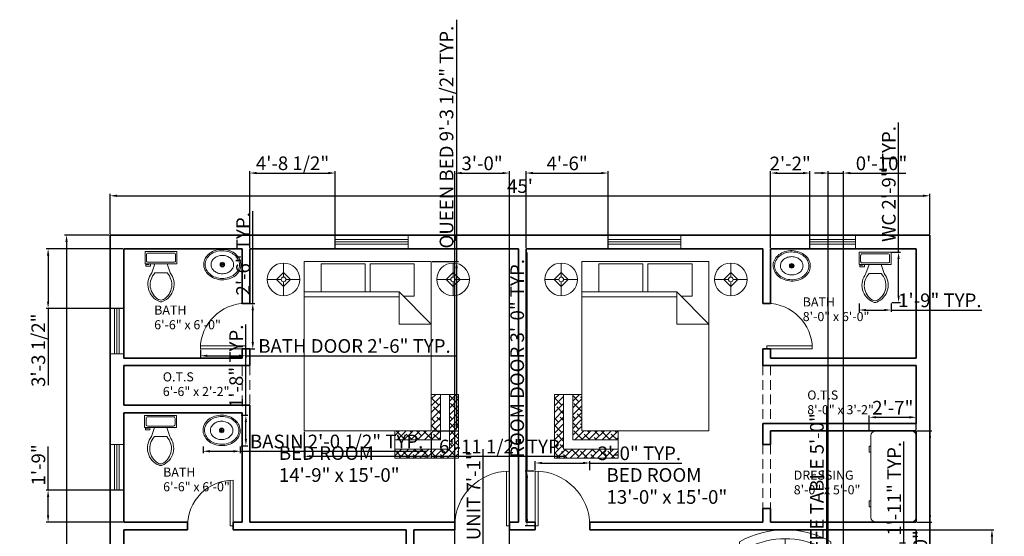
# Model space of a CAD drawing. Units: inches. Extents: x 1885 to 4781, y 1153 to 4395.
# Tile 6 of 7: x 2301 to 2950, y 2024 to 2364. Entities that reach past the tile are written whole.
import ezdxf

# ---------------------------------------------------------------- set-up
doc = ezdxf.new("R2010")
doc.units = ezdxf.units.IN
doc.linetypes.add('HIDDEN', pattern=[9.525, 6.35, -3.175])
for name, color, linetype, lineweight in [('A-ANNO-DIMS', 5, 'Continuous', 18), ('A-FURN', 8, 'Continuous', 18), ('A-WALL', 7, 'Continuous', 35)]:
    doc.layers.add(name, color=color, linetype=linetype, lineweight=lineweight)
for name, color, linetype, lineweight, true_color in [('A-AREA-IDEN', 244, 'Continuous', 18, 0x991b1e), ('A-DOOR', 11, 'Continuous', 18, 0xf27172), ('A-FLOR-FIXT', 11, 'Continuous', 18, 0xf27172), ('A-FLOR-PATT', 215, 'Continuous', 13, 0xa953a0), ('A-GLAZ', 152, 'Continuous', 18, 0x2776bb), ('A-WALL-HIDN', 11, 'HIDDEN', 18, 0xf27172)]:
    doc.layers.add(name, color=color, linetype=linetype, lineweight=lineweight, true_color=true_color)
doc.styles.get("Standard").update_dxf_attribs({"font": 'arial.ttf'})
doc.dimstyles.new('ISO-25', dxfattribs={"dimtxt": 9, "dimasz": 4.5, "dimexe": 1.25, "dimexo": 0.625, "dimtad": 1, "dimdec": 0, "dimlunit": 3, "dimtxsty": 'Standard', "dimcen": 2.5, "dimadec": 0, "dimazin": 0, "dimtfac": 1, "dimtdec": 0, "dimtmove": 0, "dimatfit": 3, "dimfxl": 1, "dimarcsym": 0})

# ---------------------------------------------------------------- blocks, each defined once
blk = doc.blocks.new('Bed - Queen')
for p, q in [((0, -80.00003), (0, 0)), ((0, 0), (59.99999, 0)), ((59.99999, 0), (59.99999, -80.00003)), ((7.99999, -1.2), (28.79998, -1.2)), ((7.99999, -14.4), (7.99999, -1.2)), ((28.79998, -1.2), (28.79998, -14.4)), ((31.19999, -1.2), (51.99999, -1.2)), ((31.19999, -14.4), (31.19999, -1.2)), ((51.99999, -1.2), (51.99999, -16.4)), ((0, -14.4), (44.8, -14.4)), ((44.8, -16.8), (0, -16.8)), ((59.99999, -29.6), (44.8, -14.4)), ((44.8, -14.4), (44.8, -29.6)), ((51.99999, -16.4), (46.79936, -16.4)), ((44.8, -29.6), (59.99999, -29.6)), ((59.99999, -80.00003), (0, -80.00003))]:
    blk.add_line(p, q)
blk = doc.blocks.new('Lamp - Table')
for p, q in [((0, 7), (0, 1)), ((-1, 0), (-7, 0)), ((0, 3), (-3, 0)), ((-3, 0), (0, -3)), ((3, 0), (0, 3)), ((0, -3), (3, 0)), ((1, 0), (7, 0)), ((0, -1), (0, -7))]:
    blk.add_line(p, q)
for radius in [7, 1]:
    blk.add_circle((0, 0), radius)
blk = doc.blocks.new('Sofa - Roundback Loveseat 5 ft.')
for p, q in [((0, -32.44198), (0, -5.99998)), ((-24, -33.99998), (-24, -11.46958)), ((24.00004, -33.99998), (24.00004, -11.46958)), ((-23.9998, -13.38178), (23.99986, -13.38178)), ((-24, -32.44198), (24.00004, -32.44198))]:
    blk.add_line(p, q)
for points in [[(-24, -33.99998), (-30, -33.99998), (-30, -7.99998)], [(30.00004, -7.99998), (30.00004, -33.99998), (24.00004, -33.99998)]]:
    blk.add_lwpolyline(points)
for centre, radius, start, end in [((0, -60.24998), 60.24998, 60.13715, 119.8628), ((0, -61.38438), 55.38444, 64.32083, 115.6792)]:
    blk.add_arc(centre, radius, start, end)
blk = doc.blocks.new('Sink - Oval top')
for p, q in [((-1, 0), (1, 0)), ((0, 1), (0, -1))]:
    blk.add_line(p, q)
for points in [[(-12.23, 0.39, 0.117634), (-11.46, -3.36, 0.104469), (-8.88, -6.8, 0.090016), (-5.08, -9.07, 0.08192), (-0.32, -10.02, 0.08192), (4.49, -9.38, 0.090016), (8.42, -7.36, 0.104469), (11.22, -4.09, 0.117634), (12.23, -0.39, 0.117634), (11.46, 3.36, 0.104469), (8.88, 6.8, 0.090016), (5.08, 9.07, 0.08192), (0.32, 10.02, 0.08192), (-4.49, 9.38, 0.090016), (-8.42, 7.36, 0.104469), (-11.22, 4.09, 0.117634)], [(-11.29, 0.16, 0.118622), (-10.52, -3.25, 0.104678), (-8.07, -6.36, 0.089562), (-4.54, -8.37, 0.081185), (-0.13, -9.15, 0.081185), (4.3, -8.49, 0.089562), (7.89, -6.58, 0.104678), (10.42, -3.55, 0.118622), (11.29, -0.16, 0.118622), (10.52, 3.25, 0.104678), (8.07, 6.36, 0.089562), (4.54, 8.37, 0.081185), (0.13, 9.15, 0.081185), (-4.3, 8.49, 0.089562), (-7.89, 6.58, 0.104678), (-10.42, 3.55, 0.118622)], [(-7.42, 0.08, 0.118283), (-6.91, -2.17, 0.104607), (-5.29, -4.21, 0.089718), (-2.97, -5.53, 0.081436), (-0.07, -6.04, 0.081436), (2.84, -5.59, 0.089718), (5.2, -4.33, 0.104607), (6.86, -2.32, 0.118283), (7.42, -0.08, 0.118283), (6.91, 2.17, 0.104607), (5.29, 4.21, 0.089718), (2.97, 5.53, 0.081436), (0.07, 6.04, 0.081436), (-2.84, 5.59, 0.089718), (-5.2, 4.33, 0.104607), (-6.86, 2.32, 0.118283)]]:
    blk.add_lwpolyline(points, format="xyb", close=True)
for radius in [1.5, 1]:
    blk.add_circle((0, 0), radius)
blk = doc.blocks.new('Toilet - top')
for p, q in [((9.5, -6), (9.5, -2)), ((-10, -8.5), (-8, -8.5)), ((-10, -9.5), (-10, -8.5)), ((-7, -9.5), (-10, -9.5)), ((-8, -8.5), (-8, -8)), ((-7, -8), (-7, -9.5)), ((-4, -8), (-6, -14)), ((4, -8), (6, -14)), ((4, -14), (-4, -14))]:
    blk.add_line(p, q)
blk.add_lwpolyline([(10.5, -8), (10.5, 0), (-10.5, 0), (-10.5, -8)], close=True)
for points in [[(-9.5, -2), (-9.5, -6)], [(8.5, -1), (-8.5, -1)], [(-8.5, -7), (8.5, -7)]]:
    blk.add_lwpolyline(points)
for centre, radius, start, end in [((-8.62, -1.88), 0.884, 81.8699, 188.1301), ((-8.62, -6.12), 0.884, 171.8699, 278.1301), ((8.62, -1.88), 0.884, 351.8699, 98.1301), ((8.62, -6.12), 0.884, 261.8699, 8.1301), ((3.52, -21.58), 12.17, 141.46911, 247.97143), ((4.2, -21.82), 11.33, 136.36773, 238.94682), ((-3.52, -21.58), 12.17, 292.02843, 38.53071), ((-4.2, -21.82), 11.33, 301.05301, 43.63209), ((0, -27.88), 4, 245.73182, 294.26817), ((0, -29), 4, 254.86053, 285.13947)]:
    blk.add_arc(centre, radius, start, end)
blk = doc.blocks.new('Desk - 30 x 60 in.')
for p, q in [((-26.999995, 0), (26.999995, 0)), ((-29.999995, -27), (-29.999995, -3)), ((29.999995, -3), (29.999995, -27)), ((26.999995, -30), (-26.999995, -30)), ((-20.000005, -30), (-20.000005, -31)), ((-20.000005, -31), (-16.000005, -31)), ((-16.000005, -31), (-16.000005, -30)), ((15.999995, -31), (15.999995, -30)), ((19.999995, -31), (15.999995, -31)), ((19.999995, -30), (19.999995, -31))]:
    blk.add_line(p, q)
for centre, start, end in [((-26.499995, -3.5), 98.1301, 171.8699), ((26.499995, -3.5), 8.130102, 81.8699), ((-26.499995, -26.5), 188.1301, 261.8699), ((26.499995, -26.5), 278.1301, 351.8699)]:
    blk.add_arc(centre, 3.535534, start, end)
blk = doc.blocks.new('*D25')
at = {"layer": 'A-ANNO-DIMS', "color": 0, "lineweight": -2, "transparency": 16777216}
for p, q in [((2360.91, 2223.05), (2360.91, 2249.5)), ((2365.41, 2248.25), (2896.41, 2248.25)), ((2900.91, 2223.05), (2900.91, 2249.5))]:
    blk.add_line(p, q, dxfattribs=at)
at = {"layer": 'A-ANNO-DIMS', "color": 0, "transparency": 16777216}
for points in [[(2365.41, 2249), (2365.41, 2247.5), (2360.91, 2248.25)], [(2896.41, 2249), (2896.41, 2247.5), (2900.91, 2248.25)]]:
    blk.add_solid(points, dxfattribs=at)
at = {"layer": 'Defpoints', "color": 0, "transparency": 16777216}
for p in [(2900.91, 2248.25), (2360.91, 2222.42), (2900.91, 2222.42)]:
    blk.add_point(p, dxfattribs=at)
at = {"layer": 'A-ANNO-DIMS', "color": 0, "transparency": 16777216, "insert": (2630.91, 2253.46), "char_height": 9, "attachment_point": 5}
blk.add_mtext("45'", dxfattribs=at)
blk = doc.blocks.new('*D26')
at = {"layer": 'A-ANNO-DIMS', "color": 0, "lineweight": -2, "transparency": 16777216}
for p, q in [((2360.28, 2222.42), (2331.02, 2222.42)), ((2332.27, 2217.92), (2332.27, 1493.92)), ((2360.28, 1489.42), (2331.02, 1489.42))]:
    blk.add_line(p, q, dxfattribs=at)
at = {"layer": 'A-ANNO-DIMS', "color": 0, "transparency": 16777216}
for points in [[(2331.52, 2217.92), (2333.02, 2217.92), (2332.27, 2222.42)], [(2331.52, 1493.92), (2333.02, 1493.92), (2332.27, 1489.42)]]:
    blk.add_solid(points, dxfattribs=at)
at = {"layer": 'Defpoints', "color": 0, "transparency": 16777216}
for p in [(2360.91, 2222.42), (2332.27, 1489.42), (2360.91, 1489.42)]:
    blk.add_point(p, dxfattribs=at)
at = {"layer": 'A-ANNO-DIMS', "color": 0, "transparency": 16777216, "insert": (2327.04, 1855.92), "char_height": 9, "attachment_point": 5, "rotation": 90}
blk.add_mtext('61\'-1"', dxfattribs=at)
blk = doc.blocks.new('WIN-48IN')
for p, q in [((0, 9), (48, 9)), ((0, 0), (0, 9)), ((48, 9), (48, 0)), ((0, 6), (48, 6)), ((0, 4.5), (48, 4.5)), ((0, 3), (48, 3)), ((48, 0), (0, 0))]:
    blk.add_line(p, q)
blk = doc.blocks.new('WIN-30IN')
for p, q in [((0, 0), (0, 30)), ((0, 30), (9, 30)), ((3, 0), (3, 30)), ((4.5, 0), (4.5, 30)), ((6, 0), (6, 30)), ((9, 30), (9, 0)), ((9, 0), (0, 0))]:
    blk.add_line(p, q)
blk = doc.blocks.new('DOOR-SWING-30IN')
for p, q in [((0, 2), (30, 2)), ((30, 0), (30, 2)), ((0, 0), (30, 0))]:
    blk.add_line(p, q)
blk.add_arc((30, 0), 30, 90, 180)
blk = doc.blocks.new('DOOR-SWING-36IN')
for p, q in [((0, 36), (0, 0)), ((2, 36), (2, 0)), ((0, 0), (2, 0))]:
    blk.add_line(p, q)
blk.add_arc((0, 0), 36, 0, 90)
blk = doc.blocks.new('RUG-CORNER-42IN')
for p, q in [((24, 18), (24, 42)), ((24, 42), (42, 42)), ((30, 42), (30, 12)), ((36, 42), (36, 6)), ((42, 42), (42, 0)), ((0, 0), (0, 18)), ((24, 18), (0, 18)), ((30, 12), (0, 12)), ((36, 6), (0, 6)), ((42, 0), (0, 0))]:
    blk.add_line(p, q)
blk = doc.blocks.new('*D36')
at = {"layer": 'A-ANNO-DIMS', "color": 0, "lineweight": -2, "transparency": 16777216}
for p, q in [((2883.59, 2019.7), (2883.59, 2086.45)), ((2880.79, 2019.7), (2884.84, 2019.7)), ((2883.59, 2001.36), (2883.59, 2015.2)), ((2880.79, 1996.86), (2884.84, 1996.86))]:
    blk.add_line(p, q, dxfattribs=at)
at = {"layer": 'A-ANNO-DIMS', "color": 0, "transparency": 16777216}
for points in [[(2882.84, 2015.2), (2884.34, 2015.2), (2883.59, 2019.7)], [(2882.84, 2001.36), (2884.34, 2001.36), (2883.59, 1996.86)]]:
    blk.add_solid(points, dxfattribs=at)
at = {"layer": 'Defpoints', "color": 0, "transparency": 16777216}
for p in [(2880.17, 2019.7), (2883.59, 2019.7), (2880.17, 1996.86)]:
    blk.add_point(p, dxfattribs=at)
at = {"layer": 'A-ANNO-DIMS', "color": 0, "transparency": 16777216, "insert": (2878.45, 2055.33), "char_height": 9, "attachment_point": 5, "rotation": 90}
blk.add_mtext('1\'-11" TYP.', dxfattribs=at)
blk = doc.blocks.new('*D41')
at = {"layer": 'A-ANNO-DIMS', "color": 0, "lineweight": -2, "transparency": 16777216}
for p, q in [((2880.21, 2211.04), (2880.21, 2296.46)), ((2875.87, 2211.04), (2881.46, 2211.04)), ((2880.21, 2182.49), (2880.21, 2206.54)), ((2875.87, 2177.99), (2881.46, 2177.99))]:
    blk.add_line(p, q, dxfattribs=at)
at = {"layer": 'A-ANNO-DIMS', "color": 0, "transparency": 16777216}
for points in [[(2879.46, 2206.54), (2880.96, 2206.54), (2880.21, 2211.04)], [(2879.46, 2182.49), (2880.96, 2182.49), (2880.21, 2177.99)]]:
    blk.add_solid(points, dxfattribs=at)
at = {"layer": 'Defpoints', "color": 0, "transparency": 16777216}
for p in [(2875.25, 2211.04), (2880.21, 2211.04), (2875.25, 2177.99)]:
    blk.add_point(p, dxfattribs=at)
at = {"layer": 'A-ANNO-DIMS', "color": 0, "transparency": 16777216, "insert": (2874.93, 2256), "char_height": 9, "attachment_point": 5, "rotation": 90}
blk.add_mtext('WC 2\'-9" TYP.', dxfattribs=at)
blk = doc.blocks.new('*D42')
at = {"layer": 'A-ANNO-DIMS', "color": 0, "lineweight": -2, "transparency": 16777216}
for p, q in [((2854.25, 2177.37), (2854.25, 2171.79)), ((2858.75, 2173.04), (2870.75, 2173.04)), ((2875.25, 2177.37), (2875.25, 2171.79)), ((2875.25, 2173.04), (2935.01, 2173.04))]:
    blk.add_line(p, q, dxfattribs=at)
at = {"layer": 'A-ANNO-DIMS', "color": 0, "transparency": 16777216}
for points in [[(2858.75, 2173.79), (2858.75, 2172.29), (2854.25, 2173.04)], [(2870.75, 2173.79), (2870.75, 2172.29), (2875.25, 2173.04)]]:
    blk.add_solid(points, dxfattribs=at)
at = {"layer": 'Defpoints', "color": 0, "transparency": 16777216}
for p in [(2854.25, 2177.99), (2875.25, 2177.99), (2875.25, 2173.04)]:
    blk.add_point(p, dxfattribs=at)
at = {"layer": 'A-ANNO-DIMS', "color": 0, "transparency": 16777216, "insert": (2907.38, 2178.26), "char_height": 9, "attachment_point": 5}
blk.add_mtext('1\'-9" TYP.', dxfattribs=at)
blk = doc.blocks.new('*D45')
at = {"layer": 'A-ANNO-DIMS', "color": 0, "lineweight": -2, "transparency": 16777216}
for p, q in [((2422.13, 2083.09), (2422.13, 2078.78)), ((2446.68, 2083.09), (2446.68, 2078.78)), ((2426.63, 2080.03), (2442.18, 2080.03)), ((2446.68, 2080.03), (2569.09, 2080.03))]:
    blk.add_line(p, q, dxfattribs=at)
at = {"layer": 'A-ANNO-DIMS', "color": 0, "transparency": 16777216}
for points in [[(2426.63, 2080.78), (2426.63, 2079.28), (2422.13, 2080.03)], [(2442.18, 2080.78), (2442.18, 2079.28), (2446.68, 2080.03)]]:
    blk.add_solid(points, dxfattribs=at)
at = {"layer": 'Defpoints', "color": 0, "transparency": 16777216}
for p in [(2422.13, 2083.71), (2446.68, 2083.71), (2446.68, 2080.03)]:
    blk.add_point(p, dxfattribs=at)
at = {"layer": 'A-ANNO-DIMS', "color": 0, "transparency": 16777216, "insert": (2510.13, 2085.31), "char_height": 9, "attachment_point": 5}
blk.add_mtext('BASIN 2\'-0 1/2" TYP.', dxfattribs=at)
blk = doc.blocks.new('*D46')
at = {"layer": 'A-ANNO-DIMS', "color": 0, "lineweight": -2, "transparency": 16777216}
for p, q in [((2450.36, 2103.85), (2450.36, 2163.61)), ((2447.31, 2103.85), (2451.61, 2103.85)), ((2450.36, 2088.21), (2450.36, 2099.35)), ((2447.31, 2083.71), (2451.61, 2083.71))]:
    blk.add_line(p, q, dxfattribs=at)
at = {"layer": 'A-ANNO-DIMS', "color": 0, "transparency": 16777216}
for points in [[(2449.61, 2099.35), (2451.11, 2099.35), (2450.36, 2103.85)], [(2449.61, 2088.21), (2451.11, 2088.21), (2450.36, 2083.71)]]:
    blk.add_solid(points, dxfattribs=at)
at = {"layer": 'Defpoints', "color": 0, "transparency": 16777216}
for p in [(2446.68, 2103.85), (2450.36, 2103.85), (2446.68, 2083.71)]:
    blk.add_point(p, dxfattribs=at)
at = {"layer": 'A-ANNO-DIMS', "color": 0, "transparency": 16777216, "insert": (2445.14, 2135.98), "char_height": 9, "attachment_point": 5, "rotation": 90}
blk.add_mtext('1\'-8" TYP.', dxfattribs=at)
blk = doc.blocks.new('*D49')
at = {"layer": 'A-ANNO-DIMS', "color": 0, "lineweight": -2, "transparency": 16777216}
for p, q in [((2420.41, 2146.8), (2420.41, 2141.67)), ((2450.41, 2146.8), (2450.41, 2141.67)), ((2424.91, 2142.92), (2445.91, 2142.92)), ((2450.41, 2142.92), (2588.86, 2142.92))]:
    blk.add_line(p, q, dxfattribs=at)
at = {"layer": 'A-ANNO-DIMS', "color": 0, "transparency": 16777216}
for points in [[(2424.91, 2143.67), (2424.91, 2142.17), (2420.41, 2142.92)], [(2445.91, 2143.67), (2445.91, 2142.17), (2450.41, 2142.92)]]:
    blk.add_solid(points, dxfattribs=at)
at = {"layer": 'Defpoints', "color": 0, "transparency": 16777216}
for p in [(2420.41, 2147.42), (2450.41, 2147.42), (2450.41, 2142.92)]:
    blk.add_point(p, dxfattribs=at)
at = {"layer": 'A-ANNO-DIMS', "color": 0, "transparency": 16777216, "insert": (2521.88, 2148.2), "char_height": 9, "attachment_point": 5}
blk.add_mtext('BATH DOOR 2\'-6" TYP.', dxfattribs=at)
blk = doc.blocks.new('*D50')
at = {"layer": 'A-ANNO-DIMS', "color": 0, "lineweight": -2, "transparency": 16777216}
for p, q in [((2454.91, 2177.42), (2454.91, 2238.18)), ((2451.03, 2177.42), (2456.16, 2177.42)), ((2454.91, 2151.92), (2454.91, 2172.92)), ((2451.03, 2147.42), (2456.16, 2147.42))]:
    blk.add_line(p, q, dxfattribs=at)
at = {"layer": 'A-ANNO-DIMS', "color": 0, "transparency": 16777216}
for points in [[(2454.16, 2172.92), (2455.66, 2172.92), (2454.91, 2177.42)], [(2454.16, 2151.92), (2455.66, 2151.92), (2454.91, 2147.42)]]:
    blk.add_solid(points, dxfattribs=at)
at = {"layer": 'Defpoints', "color": 0, "transparency": 16777216}
for p in [(2450.41, 2177.42), (2454.91, 2177.42), (2450.41, 2147.42)]:
    blk.add_point(p, dxfattribs=at)
at = {"layer": 'A-ANNO-DIMS', "color": 0, "transparency": 16777216, "insert": (2449.69, 2210.05), "char_height": 9, "attachment_point": 5, "rotation": 90}
blk.add_mtext('2\'-6" TYP.', dxfattribs=at)
blk = doc.blocks.new('*D51')
at = {"layer": 'A-ANNO-DIMS', "color": 0, "lineweight": -2, "transparency": 16777216}
for p, q in [((2635.51, 2066.92), (2635.51, 2210.88)), ((2640.28, 2066.92), (2634.26, 2066.92)), ((2635.51, 2035.42), (2635.51, 2062.42)), ((2640.28, 2030.92), (2634.26, 2030.92))]:
    blk.add_line(p, q, dxfattribs=at)
at = {"layer": 'A-ANNO-DIMS', "color": 0, "transparency": 16777216}
for points in [[(2634.76, 2062.42), (2636.26, 2062.42), (2635.51, 2066.92)], [(2634.76, 2035.42), (2636.26, 2035.42), (2635.51, 2030.92)]]:
    blk.add_solid(points, dxfattribs=at)
at = {"layer": 'Defpoints', "color": 0, "transparency": 16777216}
for p in [(2635.51, 2066.92), (2640.91, 2066.92), (2640.91, 2030.92)]:
    blk.add_point(p, dxfattribs=at)
at = {"layer": 'A-ANNO-DIMS', "color": 0, "transparency": 16777216, "insert": (2630.22, 2141.15), "char_height": 9, "attachment_point": 5, "rotation": 90}
blk.add_mtext('ROOM DOOR 3\'-0" TYP.', dxfattribs=at)
blk = doc.blocks.new('*D52')
at = {"layer": 'A-ANNO-DIMS', "color": 0, "lineweight": -2, "transparency": 16777216}
for p, q in [((2640.91, 2067.55), (2640.91, 2073.57)), ((2645.41, 2072.32), (2672.41, 2072.32)), ((2676.91, 2067.55), (2676.91, 2073.57)), ((2676.91, 2072.32), (2737.51, 2072.32))]:
    blk.add_line(p, q, dxfattribs=at)
at = {"layer": 'A-ANNO-DIMS', "color": 0, "transparency": 16777216}
for points in [[(2645.41, 2073.07), (2645.41, 2071.57), (2640.91, 2072.32)], [(2672.41, 2073.07), (2672.41, 2071.57), (2676.91, 2072.32)]]:
    blk.add_solid(points, dxfattribs=at)
at = {"layer": 'Defpoints', "color": 0, "transparency": 16777216}
for p in [(2676.91, 2072.32), (2640.91, 2066.92), (2676.91, 2066.92)]:
    blk.add_point(p, dxfattribs=at)
at = {"layer": 'A-ANNO-DIMS', "color": 0, "transparency": 16777216, "insert": (2709.46, 2077.54), "char_height": 9, "attachment_point": 5}
blk.add_mtext('3\'-0" TYP.', dxfattribs=at)
blk = doc.blocks.new('*D53')
at = {"layer": 'A-ANNO-DIMS', "color": 0, "lineweight": -2, "transparency": 16777216}
for p, q in [((2589.2, 2205.07), (2589.2, 2364.19)), ((2573.09, 2205.07), (2590.45, 2205.07)), ((2589.2, 2097.97), (2589.2, 2200.57)), ((2573.09, 2093.47), (2590.45, 2093.47))]:
    blk.add_line(p, q, dxfattribs=at)
at = {"layer": 'A-ANNO-DIMS', "color": 0, "transparency": 16777216}
for points in [[(2588.45, 2200.57), (2589.95, 2200.57), (2589.2, 2205.07)], [(2588.45, 2097.97), (2589.95, 2097.97), (2589.2, 2093.47)]]:
    blk.add_solid(points, dxfattribs=at)
at = {"layer": 'Defpoints', "color": 0, "transparency": 16777216}
for p in [(2572.46, 2205.07), (2589.2, 2205.07), (2572.46, 2093.47)]:
    blk.add_point(p, dxfattribs=at)
at = {"layer": 'A-ANNO-DIMS', "color": 0, "transparency": 16777216, "insert": (2583.65, 2286.88), "char_height": 9, "attachment_point": 5, "rotation": 90}
blk.add_mtext('QUEEN BED 9\'-3 1/2" TYP.', dxfattribs=at)
blk = doc.blocks.new('*D54')
at = {"layer": 'A-ANNO-DIMS', "color": 0, "lineweight": -2, "transparency": 16777216}
for p, q in [((2488.76, 2092.84), (2488.76, 2075.48)), ((2572.46, 2092.84), (2572.46, 2075.48)), ((2493.26, 2076.73), (2567.96, 2076.73)), ((2572.46, 2076.73), (2661.08, 2076.73))]:
    blk.add_line(p, q, dxfattribs=at)
at = {"layer": 'A-ANNO-DIMS', "color": 0, "transparency": 16777216}
for points in [[(2493.26, 2077.48), (2493.26, 2075.98), (2488.76, 2076.73)], [(2567.96, 2077.48), (2567.96, 2075.98), (2572.46, 2076.73)]]:
    blk.add_solid(points, dxfattribs=at)
at = {"layer": 'Defpoints', "color": 0, "transparency": 16777216}
for p in [(2488.76, 2093.47), (2572.46, 2093.47), (2572.46, 2076.73)]:
    blk.add_point(p, dxfattribs=at)
at = {"layer": 'A-ANNO-DIMS', "color": 0, "transparency": 16777216, "insert": (2619.02, 2082.01), "char_height": 9, "attachment_point": 5}
blk.add_mtext('6\'-11 1/2" TYP.', dxfattribs=at)
blk = doc.blocks.new('*D59')
at = {"layer": 'A-ANNO-DIMS', "color": 0, "lineweight": -2, "transparency": 16777216}
for p, q in [((2832.86, 1982.01), (2832.86, 2109.39)), ((2824.49, 1982.01), (2834.11, 1982.01)), ((2832.86, 1926.51), (2832.86, 1977.51)), ((2824.49, 1922.01), (2834.11, 1922.01))]:
    blk.add_line(p, q, dxfattribs=at)
at = {"layer": 'A-ANNO-DIMS', "color": 0, "transparency": 16777216}
for points in [[(2832.11, 1977.51), (2833.61, 1977.51), (2832.86, 1982.01)], [(2832.11, 1926.51), (2833.61, 1926.51), (2832.86, 1922.01)]]:
    blk.add_solid(points, dxfattribs=at)
at = {"layer": 'Defpoints', "color": 0, "transparency": 16777216}
for p in [(2823.86, 1982.01), (2832.86, 1982.01), (2823.86, 1922.01)]:
    blk.add_point(p, dxfattribs=at)
at = {"layer": 'A-ANNO-DIMS', "color": 0, "transparency": 16777216, "insert": (2827.58, 2047.95), "char_height": 9, "attachment_point": 5, "rotation": 90}
blk.add_mtext('COFFEE TABLE 5\'-0"', dxfattribs=at)
blk = doc.blocks.new('*D65')
at = {"layer": 'A-ANNO-DIMS', "color": 0, "lineweight": -2, "transparency": 16777216}
for p, q in [((2606.72, 1976.07), (2606.72, 2081.47)), ((2594.59, 1976.07), (2607.97, 1976.07)), ((2606.72, 1895.52), (2606.72, 1971.57)), ((2594.59, 1891.02), (2607.97, 1891.02))]:
    blk.add_line(p, q, dxfattribs=at)
at = {"layer": 'A-ANNO-DIMS', "color": 0, "transparency": 16777216}
for points in [[(2605.97, 1971.57), (2607.47, 1971.57), (2606.72, 1976.07)], [(2605.97, 1895.52), (2607.47, 1895.52), (2606.72, 1891.02)]]:
    blk.add_solid(points, dxfattribs=at)
at = {"layer": 'Defpoints', "color": 0, "transparency": 16777216}
for p in [(2593.97, 1976.07), (2606.72, 1976.07), (2593.97, 1891.02)]:
    blk.add_point(p, dxfattribs=at)
at = {"layer": 'A-ANNO-DIMS', "color": 0, "transparency": 16777216, "insert": (2601.5, 2031.02), "char_height": 9, "attachment_point": 5, "rotation": 90}
blk.add_mtext('MEDIA UNIT 7\'-1"', dxfattribs=at)
blk = doc.blocks.new('*D73')
at = {"layer": 'A-ANNO-DIMS', "color": 0, "lineweight": -2, "transparency": 16777216}
for p, q in [((2892.53, 2093.42), (2902.16, 2093.42)), ((2900.91, 2088.92), (2900.91, 2037.92)), ((2892.53, 2033.42), (2902.16, 2033.42)), ((2900.91, 2033.42), (2900.91, 1966.46))]:
    blk.add_line(p, q, dxfattribs=at)
at = {"layer": 'A-ANNO-DIMS', "color": 0, "transparency": 16777216}
for points in [[(2900.16, 2088.92), (2901.66, 2088.92), (2900.91, 2093.42)], [(2900.16, 2037.92), (2901.66, 2037.92), (2900.91, 2033.42)]]:
    blk.add_solid(points, dxfattribs=at)
at = {"layer": 'Defpoints', "color": 0, "transparency": 16777216}
for p in [(2891.91, 2093.42), (2891.91, 2033.42), (2900.91, 2033.42)]:
    blk.add_point(p, dxfattribs=at)
at = {"layer": 'A-ANNO-DIMS', "color": 0, "transparency": 16777216, "insert": (2895.63, 1997.69), "char_height": 9, "attachment_point": 5, "rotation": 90}
blk.add_mtext('DESK 5\'-0"', dxfattribs=at)
blk = doc.blocks.new('*D74')
at = {"layer": 'A-ANNO-DIMS', "color": 0, "lineweight": -2, "transparency": 16777216}
for p, q in [((2860.91, 2094.05), (2860.91, 2103.67)), ((2865.41, 2102.42), (2887.41, 2102.42)), ((2891.91, 2094.05), (2891.91, 2103.67))]:
    blk.add_line(p, q, dxfattribs=at)
at = {"layer": 'A-ANNO-DIMS', "color": 0, "transparency": 16777216}
for points in [[(2865.41, 2103.17), (2865.41, 2101.67), (2860.91, 2102.42)], [(2887.41, 2103.17), (2887.41, 2101.67), (2891.91, 2102.42)]]:
    blk.add_solid(points, dxfattribs=at)
at = {"layer": 'Defpoints', "color": 0, "transparency": 16777216}
for p in [(2891.91, 2102.42), (2860.91, 2093.42), (2891.91, 2093.42)]:
    blk.add_point(p, dxfattribs=at)
at = {"layer": 'A-ANNO-DIMS', "color": 0, "transparency": 16777216, "insert": (2876.41, 2107.56), "char_height": 9, "attachment_point": 5}
blk.add_mtext('2\'-7"', dxfattribs=at)
blk = doc.blocks.new('*D79')
at = {"layer": 'A-ANNO-DIMS', "color": 0, "lineweight": -2, "transparency": 16777216}
for p, q in [((2452.91, 2214.05), (2452.91, 2264.47)), ((2457.41, 2263.22), (2504.75, 2263.22)), ((2509.25, 2214.05), (2509.25, 2264.47))]:
    blk.add_line(p, q, dxfattribs=at)
at = {"layer": 'A-ANNO-DIMS', "color": 0, "transparency": 16777216}
for points in [[(2457.41, 2263.97), (2457.41, 2262.47), (2452.91, 2263.22)], [(2504.75, 2263.97), (2504.75, 2262.47), (2509.25, 2263.22)]]:
    blk.add_solid(points, dxfattribs=at)
at = {"layer": 'Defpoints', "color": 0, "transparency": 16777216}
for p in [(2509.25, 2263.22), (2452.91, 2213.42), (2509.25, 2213.42)]:
    blk.add_point(p, dxfattribs=at)
at = {"layer": 'A-ANNO-DIMS', "color": 0, "transparency": 16777216, "insert": (2481.08, 2268.5), "char_height": 9, "attachment_point": 5}
blk.add_mtext('4\'-8 1/2"', dxfattribs=at)
blk = doc.blocks.new('*D80')
at = {"layer": 'A-ANNO-DIMS', "color": 0, "lineweight": -2, "transparency": 16777216}
for p, q in [((2634.91, 2214.05), (2634.91, 2264.47)), ((2639.41, 2263.22), (2684.41, 2263.22)), ((2688.91, 2214.05), (2688.91, 2264.47))]:
    blk.add_line(p, q, dxfattribs=at)
at = {"layer": 'A-ANNO-DIMS', "color": 0, "transparency": 16777216}
for points in [[(2639.41, 2263.97), (2639.41, 2262.47), (2634.91, 2263.22)], [(2684.41, 2263.97), (2684.41, 2262.47), (2688.91, 2263.22)]]:
    blk.add_solid(points, dxfattribs=at)
at = {"layer": 'Defpoints', "color": 0, "transparency": 16777216}
for p in [(2688.91, 2263.22), (2634.91, 2213.42), (2688.91, 2213.42)]:
    blk.add_point(p, dxfattribs=at)
at = {"layer": 'A-ANNO-DIMS', "color": 0, "transparency": 16777216, "insert": (2661.91, 2268.44), "char_height": 9, "attachment_point": 5}
blk.add_mtext('4\'-6"', dxfattribs=at)
blk = doc.blocks.new('*D81')
at = {"layer": 'A-ANNO-DIMS', "color": 0, "lineweight": -2, "transparency": 16777216}
for p, q in [((2795.91, 2214.05), (2795.91, 2264.47)), ((2800.41, 2263.22), (2817.29, 2263.22)), ((2821.79, 2214.05), (2821.79, 2264.47))]:
    blk.add_line(p, q, dxfattribs=at)
at = {"layer": 'A-ANNO-DIMS', "color": 0, "transparency": 16777216}
for points in [[(2800.41, 2263.97), (2800.41, 2262.47), (2795.91, 2263.22)], [(2817.29, 2263.97), (2817.29, 2262.47), (2821.79, 2263.22)]]:
    blk.add_solid(points, dxfattribs=at)
at = {"layer": 'Defpoints', "color": 0, "transparency": 16777216}
for p in [(2821.79, 2263.22), (2795.91, 2213.42), (2821.79, 2213.42)]:
    blk.add_point(p, dxfattribs=at)
at = {"layer": 'A-ANNO-DIMS', "color": 0, "transparency": 16777216, "insert": (2808.85, 2268.36), "char_height": 9, "attachment_point": 5}
blk.add_mtext('2\'-2"', dxfattribs=at)
blk = doc.blocks.new('*D86')
at = {"layer": 'A-ANNO-DIMS', "color": 0, "lineweight": -2, "transparency": 16777216}
for p, q in [((2320.11, 2054.42), (2320.11, 2083.25)), ((2369.28, 2054.42), (2318.86, 2054.42)), ((2320.11, 2037.92), (2320.11, 2049.92)), ((2369.28, 2033.42), (2318.86, 2033.42))]:
    blk.add_line(p, q, dxfattribs=at)
at = {"layer": 'A-ANNO-DIMS', "color": 0, "transparency": 16777216}
for points in [[(2319.36, 2049.92), (2320.86, 2049.92), (2320.11, 2054.42)], [(2319.36, 2037.92), (2320.86, 2037.92), (2320.11, 2033.42)]]:
    blk.add_solid(points, dxfattribs=at)
at = {"layer": 'Defpoints', "color": 0, "transparency": 16777216}
for p in [(2320.11, 2054.42), (2369.91, 2054.42), (2369.91, 2033.42)]:
    blk.add_point(p, dxfattribs=at)
at = {"layer": 'A-ANNO-DIMS', "color": 0, "transparency": 16777216, "insert": (2314.89, 2071.08), "char_height": 9, "attachment_point": 5, "rotation": 90}
blk.add_mtext('1\'-9"', dxfattribs=at)
blk = doc.blocks.new('*D87')
at = {"layer": 'A-ANNO-DIMS', "color": 0, "lineweight": -2, "transparency": 16777216}
for p, q in [((2369.28, 2213.42), (2318.86, 2213.42)), ((2320.11, 2208.92), (2320.11, 2178.63)), ((2369.28, 2174.13), (2318.86, 2174.13)), ((2320.11, 2174.13), (2320.11, 2123.49))]:
    blk.add_line(p, q, dxfattribs=at)
at = {"layer": 'A-ANNO-DIMS', "color": 0, "transparency": 16777216}
for points in [[(2319.36, 2208.92), (2320.86, 2208.92), (2320.11, 2213.42)], [(2319.36, 2178.63), (2320.86, 2178.63), (2320.11, 2174.13)]]:
    blk.add_solid(points, dxfattribs=at)
at = {"layer": 'Defpoints', "color": 0, "transparency": 16777216}
for p in [(2369.91, 2213.42), (2320.11, 2174.13), (2369.91, 2174.13)]:
    blk.add_point(p, dxfattribs=at)
at = {"layer": 'A-ANNO-DIMS', "color": 0, "transparency": 16777216, "insert": (2314.83, 2146.56), "char_height": 9, "attachment_point": 5, "rotation": 90}
blk.add_mtext('3\'-3 1/2"', dxfattribs=at)
blk = doc.blocks.new('*D88')
at = {"layer": 'A-ANNO-DIMS', "color": 0, "lineweight": -2, "transparency": 16777216}
for p, q in [((2892.53, 2028.42), (2942.96, 2028.42)), ((2941.71, 2023.92), (2941.71, 2007.32)), ((2892.53, 2002.82), (2942.96, 2002.82)), ((2941.71, 2002.82), (2941.71, 1952.02))]:
    blk.add_line(p, q, dxfattribs=at)
at = {"layer": 'A-ANNO-DIMS', "color": 0, "transparency": 16777216}
for points in [[(2940.96, 2023.92), (2942.46, 2023.92), (2941.71, 2028.42)], [(2940.96, 2007.32), (2942.46, 2007.32), (2941.71, 2002.82)]]:
    blk.add_solid(points, dxfattribs=at)
at = {"layer": 'Defpoints', "color": 0, "transparency": 16777216}
for p in [(2891.91, 2028.42), (2891.91, 2002.82), (2941.71, 2002.82)]:
    blk.add_point(p, dxfattribs=at)
at = {"layer": 'A-ANNO-DIMS', "color": 0, "transparency": 16777216, "insert": (2936.43, 1975.17), "char_height": 9, "attachment_point": 5, "rotation": 90}
blk.add_mtext('2\'-1 1/2"', dxfattribs=at)
blk = doc.blocks.new('*D90')
at = {"layer": 'A-ANNO-DIMS', "color": 0, "lineweight": -2, "transparency": 16777216}
for p, q in [((2587.91, 1789.05), (2587.91, 2264.47)), ((2592.41, 2263.22), (2619.41, 2263.22)), ((2623.91, 1789.05), (2623.91, 2264.47))]:
    blk.add_line(p, q, dxfattribs=at)
at = {"layer": 'A-ANNO-DIMS', "color": 0, "transparency": 16777216}
for points in [[(2592.41, 2263.97), (2592.41, 2262.47), (2587.91, 2263.22)], [(2619.41, 2263.97), (2619.41, 2262.47), (2623.91, 2263.22)]]:
    blk.add_solid(points, dxfattribs=at)
at = {"layer": 'Defpoints', "color": 0, "transparency": 16777216}
for p in [(2623.91, 2263.22), (2587.91, 1788.42), (2623.91, 1788.42)]:
    blk.add_point(p, dxfattribs=at)
at = {"layer": 'A-ANNO-DIMS', "color": 0, "transparency": 16777216, "insert": (2605.91, 2268.44), "char_height": 9, "attachment_point": 5}
blk.add_mtext('3\'-0"', dxfattribs=at)
blk = doc.blocks.new('*D92')
at = {"layer": 'A-ANNO-DIMS', "color": 0, "lineweight": -2, "transparency": 16777216}
for p, q in [((2829.41, 2263.22), (2824.91, 2263.22)), ((2833.91, 1724.05), (2833.91, 2264.47)), ((2833.91, 2263.22), (2843.91, 2263.22)), ((2843.91, 1724.05), (2843.91, 2264.47)), ((2848.41, 2263.22), (2885.07, 2263.22))]:
    blk.add_line(p, q, dxfattribs=at)
at = {"layer": 'A-ANNO-DIMS', "color": 0, "transparency": 16777216}
for points in [[(2829.41, 2263.97), (2829.41, 2262.47), (2833.91, 2263.22)], [(2848.41, 2263.97), (2848.41, 2262.47), (2843.91, 2263.22)]]:
    blk.add_solid(points, dxfattribs=at)
at = {"layer": 'Defpoints', "color": 0, "transparency": 16777216}
for p in [(2843.91, 2263.22), (2833.91, 1723.42), (2843.91, 1723.42)]:
    blk.add_point(p, dxfattribs=at)
at = {"layer": 'A-ANNO-DIMS', "color": 0, "transparency": 16777216, "insert": (2868.99, 2268.44), "char_height": 9, "attachment_point": 5}
blk.add_mtext('0\'-10"', dxfattribs=at)

msp = doc.modelspace()

# ---------------------------------------------------------------- hatches: boundary and pattern name
at = {"layer": 'A-FLOR-PATT'}
h = msp.add_hatch(dxfattribs=at)
h.set_pattern_fill('ANSI38', color=256)
h.paths.add_polyline_path([(2578.46, 2117.47), (2572.46, 2117.47), (2572.46, 2093.47), (2548.46, 2093.47), (2548.46, 2087.47), (2578.46, 2087.47)], flags=17)
h.paths.add_polyline_path([(2590.46, 2117.47), (2584.46, 2117.47), (2584.46, 2081.47), (2548.46, 2081.47), (2548.46, 2075.47), (2590.46, 2075.47)])
h = msp.add_hatch(dxfattribs=at)
h.set_pattern_fill('ANSI38', color=256)
h.set_pattern_definition([(45, (63.172, 0), (-2.245064, 2.245064), []), (135, (63.172, 0), (-6.735192, 2.245064), [7.9375, -4.7625])])
h.paths.add_polyline_path([(2665.63, 2117.47), (2671.63, 2117.47), (2671.63, 2093.47), (2695.63, 2093.47), (2695.63, 2087.47), (2665.63, 2087.47)], flags=17)
h.paths.add_polyline_path([(2653.63, 2117.47), (2659.63, 2117.47), (2659.63, 2081.47), (2695.63, 2081.47), (2695.63, 2075.47), (2653.63, 2075.47)])

# ---------------------------------------------------------------- linework, layer by layer
at = {"layer": 'A-FURN'}
for p, q in [((2590.46, 2117.47), (2572.46, 2117.47)), ((2578.46, 2087.47), (2578.46, 2117.47)), ((2584.46, 2081.47), (2584.46, 2117.47)), ((2590.46, 2075.47), (2590.46, 2117.47)), ((2572.46, 2093.47), (2548.46, 2093.47)), ((2548.46, 2093.47), (2548.46, 2075.47)), ((2548.46, 2087.47), (2578.46, 2087.47)), ((2548.46, 2081.47), (2584.46, 2081.47)), ((2548.46, 2075.47), (2590.46, 2075.47))]:
    msp.add_line(p, q, dxfattribs=at)
at = {"layer": 'A-WALL'}
for p, q in [((2360.91, 2222.42), (2360.91, 1489.42)), ((2360.91, 2222.42), (2900.91, 2222.42)), ((2900.91, 2222.42), (2900.91, 1489.42)), ((2369.91, 2213.42), (2369.91, 2141.42)), ((2369.91, 2213.42), (2447.91, 2213.42)), ((2447.91, 2213.42), (2447.91, 2177.42)), ((2452.91, 2213.42), (2452.91, 2177.42)), ((2452.91, 2213.42), (2629.91, 2213.42)), ((2629.91, 2213.42), (2629.91, 2033.42)), ((2634.91, 2213.42), (2634.91, 2033.42)), ((2634.91, 2213.42), (2790.91, 2213.42)), ((2790.91, 2213.42), (2790.91, 2177.42)), ((2795.91, 2213.42), (2795.91, 2177.42)), ((2795.91, 2213.42), (2891.91, 2213.42)), ((2891.91, 2213.42), (2891.91, 2141.42)), ((2447.91, 2177.42), (2452.91, 2177.42)), ((2790.91, 2177.42), (2795.91, 2177.42)), ((2447.91, 2147.42), (2452.91, 2147.42)), ((2447.91, 2147.42), (2447.91, 2141.42)), ((2452.91, 2147.42), (2452.91, 2136.42)), ((2790.91, 2147.42), (2795.91, 2147.42)), ((2790.91, 2147.42), (2790.91, 2136.42)), ((2795.91, 2147.42), (2795.91, 2141.42)), ((2369.91, 2141.42), (2447.91, 2141.42)), ((2795.91, 2141.42), (2891.91, 2141.42)), ((2369.91, 2136.42), (2452.91, 2136.42)), ((2369.91, 2136.42), (2369.91, 2110.42)), ((2790.91, 2136.42), (2891.91, 2136.42)), ((2891.91, 2136.42), (2891.91, 2098.42)), ((2369.91, 2110.42), (2452.91, 2110.42)), ((2452.91, 2110.42), (2452.91, 2033.42)), ((2369.91, 2105.42), (2447.91, 2105.42)), ((2369.91, 2105.42), (2369.91, 2033.42)), ((2447.91, 2105.42), (2447.91, 2033.42)), ((2790.91, 2098.42), (2790.91, 2084.42)), ((2790.91, 2098.42), (2891.91, 2098.42)), ((2795.91, 2093.42), (2795.91, 2084.42)), ((2795.91, 2093.42), (2891.91, 2093.42)), ((2891.91, 2093.42), (2891.91, 2033.42)), ((2790.91, 2084.42), (2795.91, 2084.42)), ((2790.91, 2042.42), (2795.91, 2042.42)), ((2790.91, 2042.42), (2790.91, 2033.42)), ((2795.91, 2042.42), (2795.91, 2033.42)), ((2369.91, 2033.42), (2411.91, 2033.42)), ((2411.91, 2033.42), (2411.91, 2028.42)), ((2441.91, 2033.42), (2441.91, 2028.42)), ((2441.91, 2033.42), (2441.91, 2028.42)), ((2441.91, 2033.42), (2447.91, 2033.42)), ((2452.91, 2033.42), (2587.91, 2033.42)), ((2587.91, 2033.42), (2587.91, 2028.42)), ((2623.91, 2033.42), (2623.91, 2028.42)), ((2623.91, 2033.42), (2629.91, 2033.42)), ((2634.91, 2033.42), (2640.91, 2033.42)), ((2640.91, 2033.42), (2640.91, 2028.42)), ((2676.91, 2033.42), (2676.91, 2028.42)), ((2676.91, 2033.42), (2790.91, 2033.42)), ((2795.91, 2033.42), (2891.91, 2033.42)), ((2369.91, 2028.42), (2411.91, 2028.42)), ((2369.91, 2028.42), (2369.91, 1788.42)), ((2441.91, 2028.42), (2555.91, 2028.42)), ((2555.91, 2028.42), (2555.91, 1830.42)), ((2560.91, 2028.42), (2560.91, 1830.42)), ((2560.91, 2028.42), (2587.91, 2028.42)), ((2623.91, 2028.42), (2640.91, 2028.42)), ((2676.91, 2028.42), (2891.91, 2028.42)), ((2891.91, 2028.42), (2891.91, 1675.42))]:
    msp.add_line(p, q, dxfattribs=at)
at = {"layer": 'A-WALL-HIDN'}
for p, q in [((2447.91, 2110.42), (2447.91, 2136.42)), ((2452.91, 2136.42), (2452.91, 2108.98)), ((2790.91, 2136.42), (2790.91, 2098.42)), ((2795.91, 2136.42), (2795.91, 2098.42)), ((2790.91, 2084.42), (2790.91, 2042.42)), ((2795.91, 2084.42), (2795.91, 2042.42))]:
    msp.add_line(p, q, dxfattribs=at)

# ---------------------------------------------------------------- block references
at = {"layer": 'A-DOOR'}
for name, p in [('DOOR-SWING-30IN', (2420.41, 2147.42)), ('DOOR-SWING-36IN', (2640.91, 2030.92))]:
    msp.add_blockref(name, p, dxfattribs=at)
at = {"layer": 'A-DOOR', "extrusion": (0, 0, -1), "zscale": -1}
for name, p in [('DOOR-SWING-30IN', (-2823.41, 2147.42)), ('DOOR-SWING-36IN', (-2623.91, 2030.92))]:
    msp.add_blockref(name, p, dxfattribs=at)
at = {"layer": 'A-DOOR', "extrusion": (0, 0, -1), "zscale": -1, "rotation": 270.0000000000009}
msp.add_blockref('DOOR-SWING-30IN', (-2441.91, 2060.92), dxfattribs=at)
at = {"layer": 'A-FLOR-FIXT'}
for name, p in [('Toilet - top', (2394.47, 2211.48)), ('Sink - Oval top', (2434.84, 2202.94)), ('Sink - Oval top', (2809.86, 2202.14)), ('Toilet - top', (2864.75, 2211.04)), ('Toilet - top', (2394.2, 2103.67)), ('Sink - Oval top', (2434.41, 2093.78))]:
    msp.add_blockref(name, p, dxfattribs=at)
at = {"layer": 'A-FURN'}
for name, p, xscale, yscale, zscale in [('Bed - Queen', (2488.76, 2205.07), 1.395073646196092, 1.395073646196092, 1.395073646196092), ('Bed - Queen', (2671.63, 2205.07), 1.395073646196092, 1.395073646196092, 1.395073646196092), ('Lamp - Table', (2475.18, 2193.23), 1.53498639786184, 1.53498639786184, 1.53498639786184), ('Lamp - Table', (2586.83, 2193.23), 1.53498639786184, 1.53498639786184, 1.53498639786184), ('Lamp - Table', (2658.06, 2193.23), 1.53498639786184, 1.53498639786184, 1.53498639786184), ('Lamp - Table', (2769.71, 2193.23), 1.53498639786184, 1.53498639786184, 1.53498639786184)]:
    msp.add_blockref(name, p, dxfattribs=dict(at, xscale=xscale, yscale=yscale, zscale=zscale))
for name, p, rotation in [('RUG-CORNER-42IN', (2653.63, 2117.47), 270.000000000001), ('Desk - 30 x 60 in.', (2891.91, 2063.42), 270)]:
    msp.add_blockref(name, p, dxfattribs=dict(at, rotation=rotation))
msp.add_blockref('Sofa - Roundback Loveseat 5 ft.', (2805.52, 2028.42), dxfattribs=at)
at = {"layer": 'A-GLAZ'}
for name, p in [('WIN-48IN', (2509.26, 2213.42)), ('WIN-48IN', (2688.91, 2213.42)), ('WIN-30IN', (2360.91, 2144.13)), ('WIN-30IN', (2360.91, 2054.42))]:
    msp.add_blockref(name, p, dxfattribs=at)
at = {"layer": 'A-GLAZ', "rotation": 270.0000000000044}
msp.add_blockref('WIN-30IN', (2821.79, 2222.42), dxfattribs=at)

# ---------------------------------------------------------------- texts
at = {"layer": 'A-AREA-IDEN'}
for s, height, p in [('BATH', 6, (2817.1, 2175.37)), ('BATH', 6, (2390, 2170)), ('6\'-6" x 6\'-0"', 6, (2390, 2160.36)), ('8\'-0" x 6\'-0"', 6, (2817.1, 2165.74)), ('O.T.S', 6, (2395.66, 2126.05)), ('6\'-6" x 2\'-2"', 6, (2395.66, 2116.41)), ('O.T.S', 6, (2820.07, 2114.05)), ('8\'-0" x 3\'-2"', 6, (2820.07, 2104.41)), ('BED ROOM', 9, (2472.1, 2074.38)), ('BATH', 6, (2395.88, 2063.3)), ('14\'-9" x 15\'-0"', 9, (2472.1, 2059.92)), ('BED ROOM', 9, (2687.89, 2059.92)), ('DRESSING', 6, (2811.18, 2061.32)), ('6\'-6" x 6\'-0"', 6, (2395.88, 2053.67)), ('8\'-0" x 5\'-0"', 6, (2811.18, 2051.68)), ('13\'-0" x 15\'-0"', 9, (2687.89, 2045.46))]:
    msp.add_text(s, height=height, dxfattribs=at).set_placement(p)

# ---------------------------------------------------------------- dimensions: what is measured, and where the dimension line sits
at = {"layer": 'A-ANNO-DIMS'}
for base, p1, p2, angle, text, picture, middle in [((2589.2, 2205.07), (2572.46, 2093.47), (2572.46, 2205.07), 90, 'QUEEN BED <> TYP.', '*D53', (2583.65, 2286.88)), ((2880.2066, 2211.0387), (2875.2497, 2177.9925), (2875.2497, 2211.0387), 90, 'WC <> TYP.', '*D41', (2874.9281, 2255.9976)), ((2454.91, 2177.42), (2450.41, 2147.42), (2450.41, 2177.42), 90, '<> TYP.', '*D50', (2449.69, 2210.05)), ((2635.51, 2066.92), (2640.91, 2030.92), (2640.91, 2066.92), 90, 'ROOM DOOR <> TYP.', '*D51', (2630.22, 2141.15)), ((2450.36, 2103.85), (2446.68, 2083.71), (2446.68, 2103.85), 90, '<> TYP.', '*D46', (2445.14, 2135.98)), ((2832.86, 1982.01), (2823.86, 1922.01), (2823.86, 1982.01), 90, 'COFFEE TABLE <>', '*D59', (2827.58, 2047.95)), ((2900.91, 2033.42), (2891.91, 2093.42), (2891.91, 2033.42), 270, 'DESK <>', '*D73', (2895.63, 1997.69)), ((2883.59, 2019.7), (2880.17, 1996.86), (2880.17, 2019.7), 90, '<> TYP.', '*D36', (2878.45, 2055.33)), ((2606.7226, 1976.0689), (2593.9653, 1891.0205), (2593.9653, 1976.0689), 90, 'MEDIA UNIT <>', '*D65', (2601.5024, 2031.0193))]:
    dim = msp.add_linear_dim(base=base, p1=p1, p2=p2, angle=angle, text=text, dimstyle='ISO-25', override={"dimdec": 1, "dimlfac": 1, "dimrnd": 0, "dimzin": 1, "dimdsep": 46, "dimlunit": 4, "dimfrac": 2}, dxfattribs=at)
    dim.commit()
    dim.dimension.update_dxf_attribs({"geometry": picture, "text_midpoint": middle})
for base, p1, p2, override, picture, middle in [((2509.25, 2263.22), (2452.91, 2213.42), (2509.25, 2213.42), {"dimdec": 1, "dimlfac": 1, "dimrnd": 0, "dimzin": 1, "dimdsep": 46, "dimlunit": 4, "dimfrac": 2}, '*D79', (2481.08, 2268.5)), ((2623.91, 2263.22), (2587.91, 1788.42), (2623.91, 1788.42), {"dimdec": 1, "dimlfac": 1, "dimrnd": 0, "dimzin": 1, "dimdsep": 46, "dimlunit": 4, "dimfrac": 2}, '*D90', (2605.91, 2268.44)), ((2688.91, 2263.22), (2634.91, 2213.42), (2688.91, 2213.42), {"dimdec": 1, "dimlfac": 1, "dimrnd": 0, "dimzin": 1, "dimdsep": 46, "dimlunit": 4, "dimfrac": 2}, '*D80', (2661.91, 2268.44)), ((2821.79, 2263.22), (2795.91, 2213.42), (2821.79, 2213.42), {"dimdec": 1, "dimlfac": 1, "dimrnd": 0, "dimzin": 1, "dimdsep": 46, "dimlunit": 4, "dimfrac": 2}, '*D81', (2808.85, 2268.36)), ((2843.91, 2263.22), (2833.91, 1723.42), (2843.91, 1723.42), {"dimdec": 1, "dimlfac": 1, "dimrnd": 0, "dimzin": 1, "dimdsep": 46, "dimlunit": 4, "dimfrac": 2}, '*D92', (2868.99, 2268.44)), ((2900.91, 2248.25), (2360.91, 2222.42), (2900.91, 2222.42), {"dimclrd": 0, "dimclre": 0, "dimclrt": 0}, '*D25', (2630.91, 2253.46)), ((2891.91, 2102.42), (2860.91, 2093.42), (2891.91, 2093.42), {"dimdec": 1, "dimlfac": 1, "dimrnd": 0, "dimzin": 1, "dimdsep": 46, "dimlunit": 4, "dimfrac": 2}, '*D74', (2876.41, 2107.56))]:
    dim = msp.add_linear_dim(base=base, p1=p1, p2=p2, dimstyle='ISO-25', override=override, dxfattribs=at)
    dim.commit()
    dim.dimension.update_dxf_attribs({"geometry": picture, "text_midpoint": middle})
for base, p1, p2, override, picture, middle in [((2332.27, 1489.42), (2360.91, 2222.42), (2360.91, 1489.42), {"dimclrd": 0, "dimclre": 0, "dimclrt": 0}, '*D26', (2327.04, 1855.92)), ((2320.11, 2174.13), (2369.91, 2213.42), (2369.91, 2174.13), {"dimdec": 1, "dimlfac": 1, "dimrnd": 0, "dimzin": 1, "dimdsep": 46, "dimlunit": 4, "dimfrac": 2}, '*D87', (2314.83, 2146.56)), ((2320.11, 2054.42), (2369.91, 2033.42), (2369.91, 2054.42), {"dimdec": 1, "dimlfac": 1, "dimrnd": 0, "dimzin": 1, "dimdsep": 46, "dimlunit": 4, "dimfrac": 2}, '*D86', (2314.89, 2071.08)), ((2941.71, 2002.82), (2891.91, 2028.42), (2891.91, 2002.82), {"dimdec": 1, "dimlfac": 1, "dimrnd": 0, "dimzin": 1, "dimdsep": 46, "dimlunit": 4, "dimfrac": 2}, '*D88', (2936.43, 1975.17))]:
    dim = msp.add_linear_dim(base=base, p1=p1, p2=p2, angle=90, dimstyle='ISO-25', override=override, dxfattribs=at)
    dim.commit()
    dim.dimension.update_dxf_attribs({"geometry": picture, "text_midpoint": middle})
for base, p1, p2, text, picture, middle in [((2875.25, 2173.04), (2854.25, 2177.99), (2875.25, 2177.99), '<> TYP.', '*D42', (2907.38, 2178.26)), ((2450.41, 2142.92), (2420.41, 2147.42), (2450.41, 2147.42), 'BATH DOOR <> TYP.', '*D49', (2521.88, 2148.2)), ((2446.681, 2080.0277), (2422.1301, 2083.7103), (2446.681, 2083.7103), 'BASIN <> TYP.', '*D45', (2510.1341, 2085.3062)), ((2572.46, 2076.73), (2488.76, 2093.47), (2572.46, 2093.47), '<> TYP.', '*D54', (2619.02, 2082.01)), ((2676.91, 2072.32), (2640.91, 2066.92), (2676.91, 2066.92), '<> TYP.', '*D52', (2709.46, 2077.54))]:
    dim = msp.add_linear_dim(base=base, p1=p1, p2=p2, text=text, dimstyle='ISO-25', override={"dimdec": 1, "dimlfac": 1, "dimrnd": 0, "dimzin": 1, "dimdsep": 46, "dimlunit": 4, "dimfrac": 2}, dxfattribs=at)
    dim.commit()
    dim.dimension.update_dxf_attribs({"geometry": picture, "text_midpoint": middle})

doc.saveas('drawing.dxf')
